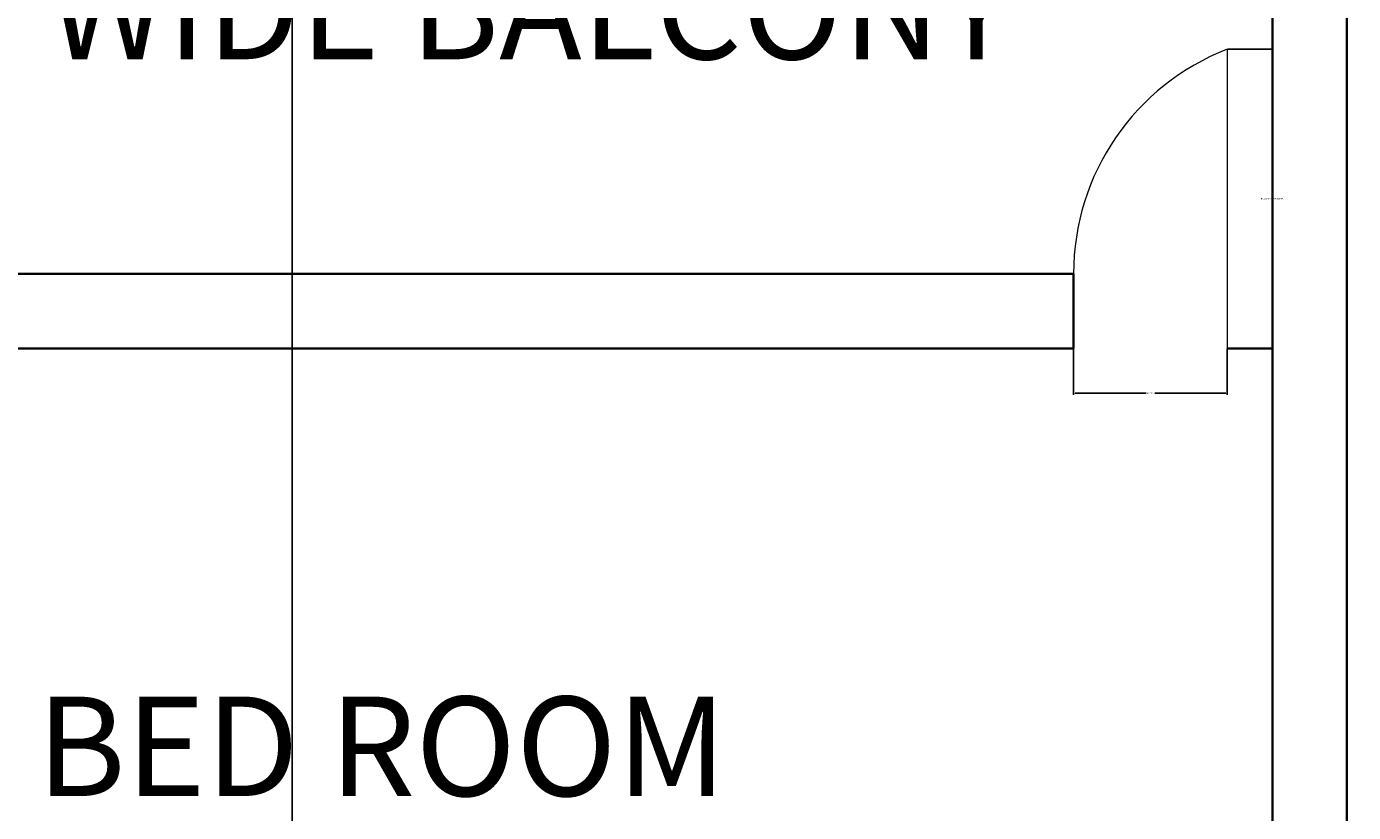
# Model space of a CAD drawing. Units: feet. Extents: x 5816 to 6644, y 25475 to 26788.
# Tile 13 of 23: x 5922 to 6082, y 26597 to 26691. Entities that reach past the tile are written whole.
import ezdxf

# ---------------------------------------------------------------- set-up
doc = ezdxf.new("R2010")
doc.units = ezdxf.units.FT
for name, color, linetype, lineweight in [('A-ANNO-DIMS', 2, 'Continuous', 13), ('A-AREA-IDEN', 7, 'Continuous', 18), ('A-DOOR', 3, 'Continuous', 18), ('A-WALL', 7, 'Continuous', 35)]:
    doc.layers.add(name, color=color, linetype=linetype, lineweight=lineweight)
doc.styles.get("Standard").update_dxf_attribs({"font": 'arial.ttf'})
doc.dimstyles.get("Standard").update_dxf_attribs({"dimtxt": 0.18, "dimasz": 0.18, "dimexe": 0.18, "dimexo": 0.0625, "dimgap": 0.09, "dimtad": 0, "dimtih": 1, "dimtoh": 1, "dimdec": 4, "dimzin": 0, "dimdsep": 46, "dimtxsty": 'Standard', "dimcen": 0.09, "dimadec": 0, "dimazin": 0, "dimtfac": 1, "dimtdec": 4, "dimtofl": 0, "dimtmove": 0, "dimatfit": 3, "dimfxl": 1, "dimtolj": 1, "dimtzin": 0, "dimarcsym": 0})

# ---------------------------------------------------------------- blocks, each defined once
blk = doc.blocks.new('DOOR-BALCONY')
blk.add_line((0, 36.11), (0, 0))
blk.add_arc((10.54, 9), 29.09, 111.2433, 180)
blk = doc.blocks.new('*D19')
at = {"layer": 'A-ANNO-DIMS', "color": 0, "lineweight": -2, "transparency": 16777216}
for p, q in [((6066.92, 26688.7), (6072.46, 26688.7)), ((6072.28, 26688.52), (6072.28, 26670.82)), ((6072.28, 26652.76), (6072.28, 26670.46)), ((6066.92, 26652.58), (6072.46, 26652.58))]:
    blk.add_line(p, q, dxfattribs=at)
at = {"layer": 'A-ANNO-DIMS', "color": 0, "transparency": 16777216}
for points in [[(6072.25, 26688.52), (6072.31, 26688.52), (6072.28, 26688.7)], [(6072.25, 26652.76), (6072.31, 26652.76), (6072.28, 26652.58)]]:
    blk.add_solid(points, dxfattribs=at)
at = {"layer": 'Defpoints', "color": 0, "transparency": 16777216}
for p in [(6066.86, 26688.7), (6072.28, 26688.7), (6066.86, 26652.58)]:
    blk.add_point(p, dxfattribs=at)
at = {"layer": 'A-ANNO-DIMS', "color": 0, "transparency": 16777216, "insert": (6072.28, 26670.64), "char_height": 0.18, "attachment_point": 5}
blk.add_mtext('\\A1;BALCONY DOOR 36 TYP.', dxfattribs=at)
blk = doc.blocks.new('*D20')
at = {"layer": 'A-ANNO-DIMS', "color": 0, "lineweight": -2, "transparency": 16777216}
for p, q in [((6048.31, 26652.52), (6048.31, 26646.99)), ((6066.86, 26652.52), (6066.86, 26646.99)), ((6048.49, 26647.17), (6057.07, 26647.17)), ((6066.68, 26647.17), (6058.11, 26647.17))]:
    blk.add_line(p, q, dxfattribs=at)
at = {"layer": 'A-ANNO-DIMS', "color": 0, "transparency": 16777216}
for points in [[(6048.49, 26647.2), (6048.49, 26647.14), (6048.31, 26647.17)], [(6066.68, 26647.2), (6066.68, 26647.14), (6066.86, 26647.17)]]:
    blk.add_solid(points, dxfattribs=at)
at = {"layer": 'Defpoints', "color": 0, "transparency": 16777216}
for p in [(6048.31, 26652.58), (6066.86, 26652.58), (6066.86, 26647.17)]:
    blk.add_point(p, dxfattribs=at)
at = {"layer": 'A-ANNO-DIMS', "color": 0, "transparency": 16777216, "insert": (6057.59, 26647.17), "char_height": 0.18, "attachment_point": 5}
blk.add_mtext('\\A1;19 TYP.', dxfattribs=at)
blk = doc.blocks.new('*D58')
at = {"layer": 'A-ANNO-DIMS', "color": 0, "lineweight": -2, "transparency": 16777216}
for p, q in [((5953.98, 26168.65), (5953.98, 26787.91)), ((5954.16, 26787.73), (6030.2, 26787.73)), ((6106.8, 26787.73), (6030.76, 26787.73)), ((6106.98, 26168.71), (6106.98, 26787.91))]:
    blk.add_line(p, q, dxfattribs=at)
at = {"layer": 'A-ANNO-DIMS', "color": 0, "transparency": 16777216}
for points in [[(5954.16, 26787.76), (5954.16, 26787.7), (5953.98, 26787.73)], [(6106.8, 26787.76), (6106.8, 26787.7), (6106.98, 26787.73)]]:
    blk.add_solid(points, dxfattribs=at)
at = {"layer": 'Defpoints', "color": 0, "transparency": 16777216}
for p in [(6106.98, 26787.73), (5953.98, 26168.58), (6106.98, 26168.65)]:
    blk.add_point(p, dxfattribs=at)
at = {"layer": 'A-ANNO-DIMS', "color": 0, "transparency": 16777216, "insert": (6030.48, 26787.73), "char_height": 0.18, "attachment_point": 5}
blk.add_mtext('\\A1;153', dxfattribs=at)

msp = doc.modelspace()

# ---------------------------------------------------------------- linework, layer by layer
at = {"layer": 'A-WALL'}
for p, q in [((6072.3119, 26661.5846), (6072.3119, 26726.5846)), ((6081.3119, 26661.5846), (6081.3119, 26717.5846)), ((6072.3119, 26558.5846), (6072.3119, 26668.7645)), ((6081.3119, 26558.5846), (6081.3119, 26668.7645)), ((5877.3119, 26661.5846), (6048.3119, 26661.5846)), ((6048.3119, 26652.5846), (6048.3119, 26661.5846)), ((5886.3119, 26652.5846), (6048.3119, 26652.5846)), ((6066.8616, 26652.5846), (6072.3119, 26652.5846))]:
    msp.add_line(p, q, dxfattribs=at)

# ---------------------------------------------------------------- block references
at = {"layer": 'A-DOOR'}
msp.add_blockref('DOOR-BALCONY', (6066.8616, 26652.5846), dxfattribs=at)

# ---------------------------------------------------------------- texts
at = {"layer": 'A-AREA-IDEN'}
for s, p in [('4\'8" WIDE BALCONY', (5890.3368, 26687.4804)), ('BED ROOM', (5923.1507, 26598.538))]:
    msp.add_text(s, height=12, dxfattribs=at).set_placement(p)

# ---------------------------------------------------------------- dimensions: what is measured, and where the dimension line sits
at = {"layer": 'A-ANNO-DIMS'}
dim = msp.add_linear_dim(base=(6106.9781, 26787.7346), p1=(5953.9781, 26168.5846), p2=(6106.9781, 26168.6509), dimstyle='Standard', override={"dimdec": 0, "dimlfac": 1, "dimrnd": 0, "dimzin": 0, "dimdsep": 46, "dimlunit": 2}, dxfattribs=at)
dim.commit()
dim.dimension.update_dxf_attribs({"geometry": '*D58', "text_midpoint": (6030.4781, 26787.7346)})
dim = msp.add_linear_dim(base=(6072.2785, 26688.6978), p1=(6066.8616, 26652.5846), p2=(6066.8616, 26688.6978), angle=90, text='BALCONY DOOR <> TYP.', dimstyle='Standard', override={"dimdec": 0, "dimlfac": 1, "dimrnd": 0, "dimzin": 0, "dimdsep": 46, "dimlunit": 2}, dxfattribs=at)
dim.commit()
dim.dimension.update_dxf_attribs({"geometry": '*D19', "text_midpoint": (6072.2785, 26670.6412)})
dim = msp.add_linear_dim(base=(6066.8616, 26647.1677), p1=(6048.3119, 26652.5846), p2=(6066.8616, 26652.5846), text='<> TYP.', dimstyle='Standard', override={"dimdec": 0, "dimlfac": 1, "dimrnd": 0, "dimzin": 0, "dimdsep": 46, "dimlunit": 2}, dxfattribs=at)
dim.commit()
dim.dimension.update_dxf_attribs({"geometry": '*D20', "text_midpoint": (6057.5867, 26647.1677)})

doc.saveas('drawing.dxf')
